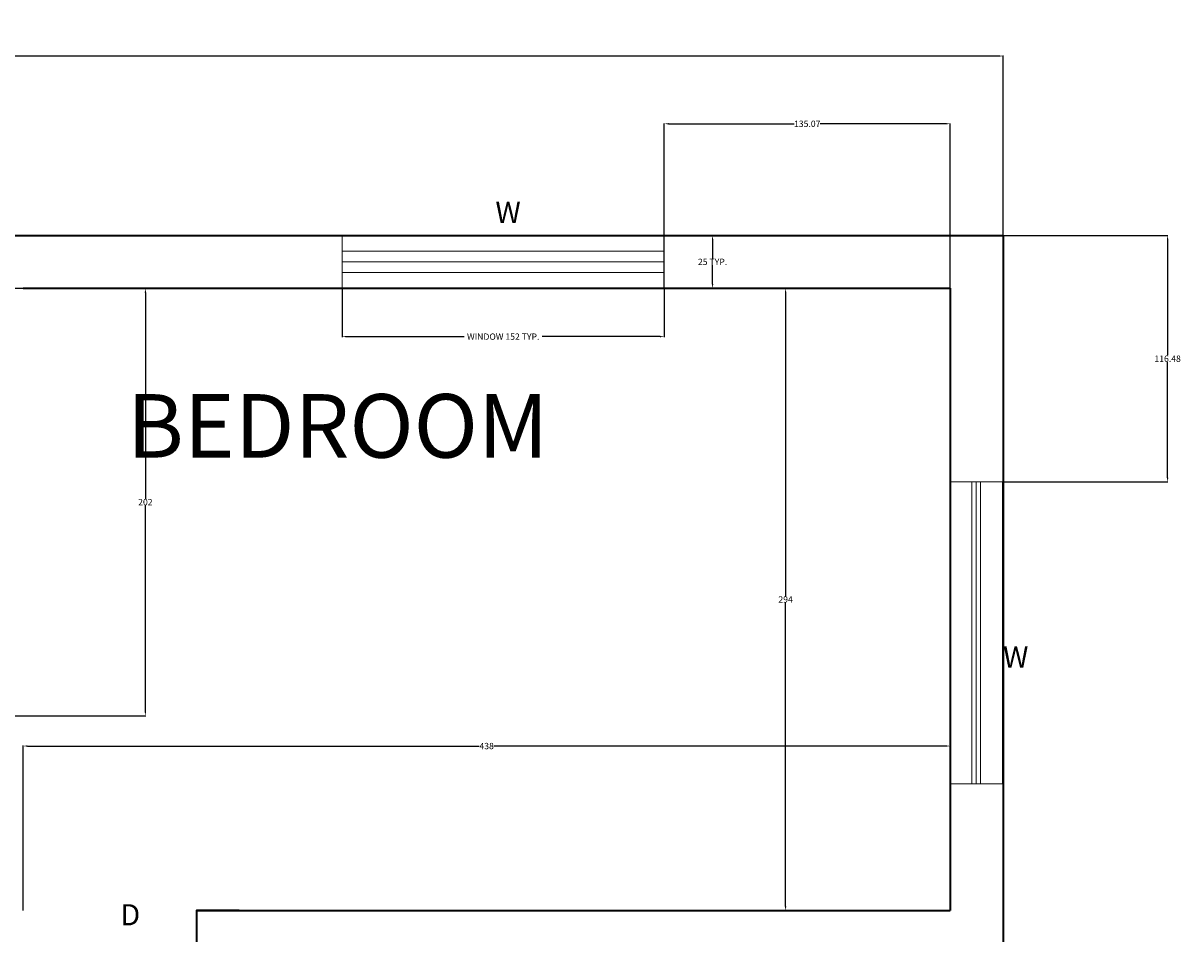
# Model space of a CAD drawing. Units: centimetres. Extents: x -121 to 3851, y -16 to 1180.
# Tile 16 of 16: x 3304 to 3851, y 582 to 1012. Entities that reach past the tile are written whole.
import ezdxf

# ---------------------------------------------------------------- set-up
doc = ezdxf.new("R2010")
doc.units = ezdxf.units.CM
doc.header["$MEASUREMENT"] = 0
for name, color, linetype, lineweight in [('A-ANNO-DIMS', 2, 'Continuous', 18), ('A-ANNO-IDEN', 3, 'Continuous', 13), ('A-AREA-IDEN', 3, 'Continuous', 18), ('A-GLAZ', 4, 'Continuous', 18), ('A-WALL', 7, 'Continuous', 35)]:
    doc.layers.add(name, color=color, linetype=linetype, lineweight=lineweight)
doc.styles.get("Standard").update_dxf_attribs({"font": 'arial.ttf'})
doc.dimstyles.get("Standard").update_dxf_attribs({"dimtxt": 3, "dimasz": 2, "dimexe": 0.18, "dimexo": 0.0625, "dimgap": 0.09, "dimtad": 0, "dimtih": 1, "dimtoh": 1, "dimdec": 0, "dimzin": 0, "dimdsep": 46, "dimtxsty": 'Standard', "dimcen": 0.09, "dimadec": 0, "dimazin": 0, "dimtfac": 1, "dimtdec": 0, "dimtofl": 0, "dimtmove": 0, "dimatfit": 3, "dimfxl": 1, "dimtolj": 1, "dimtzin": 0, "dimarcsym": 0})

# ---------------------------------------------------------------- blocks, each defined once
blk = doc.blocks.new('*D16')
at = {"layer": 'A-ANNO-DIMS', "color": 0, "lineweight": -2, "transparency": 16777216}
for p, q in [((2411.26, 911.79), (2411.26, 996.66)), ((2413.26, 996.48), (3045.8, 996.48)), ((3765.26, 996.48), (3132.73, 996.48)), ((3767.26, 911.79), (3767.26, 996.66))]:
    blk.add_line(p, q, dxfattribs=at)
at = {"layer": 'A-ANNO-DIMS', "color": 0, "transparency": 16777216}
for points in [[(2413.26, 996.81), (2413.26, 996.14), (2411.26, 996.48)], [(3765.26, 996.81), (3765.26, 996.14), (3767.26, 996.48)]]:
    blk.add_solid(points, dxfattribs=at)
at = {"layer": 'Defpoints', "color": 0, "transparency": 16777216}
for p in [(3767.26, 996.48), (2411.26, 911.72), (3767.26, 911.72)]:
    blk.add_point(p, dxfattribs=at)
at = {"layer": 'A-ANNO-DIMS', "color": 0, "transparency": 16777216, "insert": (3089.26, 996.48), "char_height": 3, "attachment_point": 5}
blk.add_mtext('\\A1;{\\H10x;1356}', dxfattribs=at)
blk = doc.blocks.new('WIN-152CM')
for p, q in [((0, 17.5), (152.19, 17.5)), ((0, 12.5), (152.19, 12.5)), ((0, 7.5), (152.19, 7.5))]:
    blk.add_line(p, q)
blk.add_lwpolyline([(0, 25), (152.19, 25), (152.19, 0), (0, 0)], close=True)
blk = doc.blocks.new('WIN-143CM')
for p, q in [((0, 14.5), (142.63, 14.5)), ((0, 12.5), (142.63, 12.5)), ((0, 10.5), (142.63, 10.5))]:
    blk.add_line(p, q)
blk.add_lwpolyline([(0, 25), (142.63, 25), (142.63, 0), (0, 0)], close=True)
blk = doc.blocks.new('*D27')
at = {"layer": 'A-ANNO-DIMS', "color": 0, "lineweight": -2, "transparency": 16777216}
for p, q in [((3455, 886.66), (3455, 863.71)), ((3607.19, 886.66), (3607.19, 863.71)), ((3457, 863.89), (3512.7, 863.89)), ((3605.19, 863.89), (3549.49, 863.89))]:
    blk.add_line(p, q, dxfattribs=at)
at = {"layer": 'A-ANNO-DIMS', "color": 0, "transparency": 16777216}
for points in [[(3457, 864.23), (3457, 863.56), (3455, 863.89)], [(3605.19, 864.23), (3605.19, 863.56), (3607.19, 863.89)]]:
    blk.add_solid(points, dxfattribs=at)
at = {"layer": 'Defpoints', "color": 0, "transparency": 16777216}
for p in [(3455, 886.72), (3607.19, 886.72), (3607.19, 863.89)]:
    blk.add_point(p, dxfattribs=at)
at = {"layer": 'A-ANNO-DIMS', "color": 0, "transparency": 16777216, "insert": (3531.09, 863.89), "char_height": 3, "attachment_point": 5}
blk.add_mtext('\\A1;WINDOW 152 TYP.', dxfattribs=at)
blk = doc.blocks.new('*D28')
at = {"layer": 'A-ANNO-DIMS', "color": 0, "lineweight": -2, "transparency": 16777216}
for p, q in [((3607.25, 911.72), (3630.2, 911.72)), ((3630.02, 909.72), (3630.02, 900.84)), ((3630.02, 888.72), (3630.02, 897.6)), ((3607.25, 886.72), (3630.2, 886.72))]:
    blk.add_line(p, q, dxfattribs=at)
at = {"layer": 'A-ANNO-DIMS', "color": 0, "transparency": 16777216}
for points in [[(3629.68, 909.72), (3630.35, 909.72), (3630.02, 911.72)], [(3629.68, 888.72), (3630.35, 888.72), (3630.02, 886.72)]]:
    blk.add_solid(points, dxfattribs=at)
at = {"layer": 'Defpoints', "color": 0, "transparency": 16777216}
for p in [(3607.19, 911.72), (3630.02, 911.72), (3607.19, 886.72)]:
    blk.add_point(p, dxfattribs=at)
at = {"layer": 'A-ANNO-DIMS', "color": 0, "transparency": 16777216, "insert": (3630.02, 899.22), "char_height": 3, "attachment_point": 5}
blk.add_mtext('\\A1;25 TYP.', dxfattribs=at)
blk = doc.blocks.new('*D69')
at = {"layer": 'A-ANNO-DIMS', "color": 0, "lineweight": -2, "transparency": 16777216}
for p, q in [((3284.33, 886.72), (3362.19, 886.72)), ((3362.01, 884.72), (3362.01, 787.34)), ((3362.01, 686.72), (3362.01, 784.1)), ((3284.33, 684.72), (3362.19, 684.72))]:
    blk.add_line(p, q, dxfattribs=at)
at = {"layer": 'A-ANNO-DIMS', "color": 0, "transparency": 16777216}
for points in [[(3361.68, 884.72), (3362.35, 884.72), (3362.01, 886.72)], [(3361.68, 686.72), (3362.35, 686.72), (3362.01, 684.72)]]:
    blk.add_solid(points, dxfattribs=at)
at = {"layer": 'Defpoints', "color": 0, "transparency": 16777216}
for p in [(3284.26, 886.72), (3284.26, 684.72), (3362.01, 684.72)]:
    blk.add_point(p, dxfattribs=at)
at = {"layer": 'A-ANNO-DIMS', "color": 0, "transparency": 16777216, "insert": (3362.01, 785.72), "char_height": 3, "attachment_point": 5}
blk.add_mtext('\\A1;202', dxfattribs=at)
blk = doc.blocks.new('*D70')
at = {"layer": 'A-ANNO-DIMS', "color": 0, "lineweight": -2, "transparency": 16777216}
for p, q in [((3767.33, 911.72), (3845.19, 911.72)), ((3845.01, 909.72), (3845.01, 855.11)), ((3845.01, 797.25), (3845.01, 851.86)), ((3767.14, 795.25), (3845.19, 795.25))]:
    blk.add_line(p, q, dxfattribs=at)
at = {"layer": 'A-ANNO-DIMS', "color": 0, "transparency": 16777216}
for points in [[(3844.68, 909.72), (3845.35, 909.72), (3845.01, 911.72)], [(3844.68, 797.25), (3845.35, 797.25), (3845.01, 795.25)]]:
    blk.add_solid(points, dxfattribs=at)
at = {"layer": 'Defpoints', "color": 0, "transparency": 16777216}
for p in [(3767.26, 911.72), (3767.07, 795.25), (3845.01, 795.25)]:
    blk.add_point(p, dxfattribs=at)
at = {"layer": 'A-ANNO-DIMS', "color": 0, "transparency": 16777216, "insert": (3845.01, 853.48), "char_height": 3, "attachment_point": 5}
blk.add_mtext('\\A1;116.48', dxfattribs=at)
blk = doc.blocks.new('*D71')
at = {"layer": 'A-ANNO-DIMS', "color": 0, "lineweight": -2, "transparency": 16777216}
for p, q in [((3607.19, 886.79), (3607.19, 964.65)), ((3609.19, 964.47), (3668.55, 964.47)), ((3740.26, 964.47), (3680.9, 964.47)), ((3742.26, 886.79), (3742.26, 964.65))]:
    blk.add_line(p, q, dxfattribs=at)
at = {"layer": 'A-ANNO-DIMS', "color": 0, "transparency": 16777216}
for points in [[(3609.19, 964.81), (3609.19, 964.14), (3607.19, 964.47)], [(3740.26, 964.81), (3740.26, 964.14), (3742.26, 964.47)]]:
    blk.add_solid(points, dxfattribs=at)
at = {"layer": 'Defpoints', "color": 0, "transparency": 16777216}
for p in [(3742.26, 964.47), (3607.19, 886.72), (3742.26, 886.72)]:
    blk.add_point(p, dxfattribs=at)
at = {"layer": 'A-ANNO-DIMS', "color": 0, "transparency": 16777216, "insert": (3674.73, 964.47), "char_height": 3, "attachment_point": 5}
blk.add_mtext('\\A1;135.07', dxfattribs=at)
blk = doc.blocks.new('*D81')
at = {"layer": 'A-ANNO-DIMS', "color": 0, "lineweight": -2, "transparency": 16777216}
for p, q in [((3304.26, 592.79), (3304.26, 670.65)), ((3306.26, 670.47), (3519.8, 670.47)), ((3740.26, 670.47), (3526.73, 670.47)), ((3742.26, 592.79), (3742.26, 670.65))]:
    blk.add_line(p, q, dxfattribs=at)
at = {"layer": 'A-ANNO-DIMS', "color": 0, "transparency": 16777216}
for points in [[(3306.26, 670.81), (3306.26, 670.14), (3304.26, 670.47)], [(3740.26, 670.81), (3740.26, 670.14), (3742.26, 670.47)]]:
    blk.add_solid(points, dxfattribs=at)
at = {"layer": 'Defpoints', "color": 0, "transparency": 16777216}
for p in [(3742.26, 670.47), (3304.26, 592.72), (3742.26, 592.72)]:
    blk.add_point(p, dxfattribs=at)
at = {"layer": 'A-ANNO-DIMS', "color": 0, "transparency": 16777216, "insert": (3523.26, 670.47), "char_height": 3, "attachment_point": 5}
blk.add_mtext('\\A1;438', dxfattribs=at)
blk = doc.blocks.new('*D82')
at = {"layer": 'A-ANNO-DIMS', "color": 0, "lineweight": -2, "transparency": 16777216}
for p, q in [((3742.2, 886.72), (3664.33, 886.72)), ((3664.51, 884.72), (3664.51, 741.34)), ((3664.51, 594.72), (3664.51, 738.1)), ((3742.2, 592.72), (3664.33, 592.72))]:
    blk.add_line(p, q, dxfattribs=at)
at = {"layer": 'A-ANNO-DIMS', "color": 0, "transparency": 16777216}
for points in [[(3664.18, 884.72), (3664.85, 884.72), (3664.51, 886.72)], [(3664.18, 594.72), (3664.85, 594.72), (3664.51, 592.72)]]:
    blk.add_solid(points, dxfattribs=at)
at = {"layer": 'Defpoints', "color": 0, "transparency": 16777216}
for p in [(3664.51, 886.72), (3742.26, 886.72), (3742.26, 592.72)]:
    blk.add_point(p, dxfattribs=at)
at = {"layer": 'A-ANNO-DIMS', "color": 0, "transparency": 16777216, "insert": (3664.51, 739.72), "char_height": 3, "attachment_point": 5}
blk.add_mtext('\\A1;294', dxfattribs=at)

msp = doc.modelspace()

# ---------------------------------------------------------------- linework, layer by layer
at = {"layer": 'A-WALL'}
for p, q in [((2736.2642, 911.7228), (3767.2642, 911.7228)), ((3767.2642, 911.7228), (3767.2642, 95.7228)), ((3304.2642, 886.7228), (3742.2642, 886.7228)), ((3742.2642, 886.7228), (3742.2642, 592.7228)), ((3386.2335, 592.7228), (3742.2642, 592.7228))]:
    msp.add_line(p, q, dxfattribs=at)
msp.add_lwpolyline([(3406.327, 592.7228), (3386.2335, 592.7228), (3386.2335, 415.7228)], dxfattribs=at)

# ---------------------------------------------------------------- block references
at = {"layer": 'A-GLAZ'}
msp.add_blockref('WIN-152CM', (3454.9993, 886.7227), dxfattribs=at)
at = {"layer": 'A-GLAZ', "rotation": 89.99999999999976}
msp.add_blockref('WIN-143CM', (3767.0732, 652.6168), dxfattribs=at)

# ---------------------------------------------------------------- texts
at = {"layer": 'A-ANNO-IDEN', "char_height": 10, "attachment_point": 1}
for s, insert in [('W', (3527.3985, 927.6121)), ('W', (3767.2642, 717.5214)), ('D', (3350.1824, 595.7422))]:
    msp.add_mtext_dynamic_manual_height_columns(s, width=55.718495, gutter_width=1, heights=[0], dxfattribs=dict(at, insert=insert))
at = {"layer": 'A-AREA-IDEN', "insert": (3353.2806, 836.7321), "char_height": 30, "attachment_point": 1}
msp.add_mtext_dynamic_manual_height_columns('BEDROOM', width=248.976965, gutter_width=1, heights=[0], dxfattribs=at)

# ---------------------------------------------------------------- dimensions: what is measured, and where the dimension line sits
at = {"layer": 'A-ANNO-DIMS'}
for base, p1, p2, text, override, picture, middle in [((3767.2642, 996.4769), (2411.2642, 911.7228), (3767.2642, 911.7228), '{\\H10x;<>}', {"dimclrd": 0, "dimclre": 0, "dimclrt": 0}, '*D16', (3089.2642, 996.4769)), ((3607.1897, 863.8943), (3454.9995, 886.7228), (3607.1897, 886.7228), 'WINDOW <> TYP.', {"dimdec": 0, "dimlfac": 1, "dimrnd": 0, "dimzin": 0, "dimdsep": 46, "dimlunit": 2}, '*D27', (3531.0946, 863.8943))]:
    dim = msp.add_linear_dim(base=base, p1=p1, p2=p2, text=text, dimstyle='Standard', override=override, dxfattribs=at)
    dim.commit()
    dim.dimension.update_dxf_attribs({"geometry": picture, "text_midpoint": middle})
for base, p1, p2, override, picture, middle in [((3742.2642, 964.4728), (3607.1897, 886.7228), (3742.2642, 886.7228), {"dimdec": 2, "dimlfac": 1, "dimrnd": 0, "dimzin": 0, "dimdsep": 46, "dimlunit": 2}, '*D71', (3674.727, 964.4728)), ((3742.2642, 670.4728), (3304.2642, 592.7228), (3742.2642, 592.7228), {"dimdec": 0, "dimlfac": 1, "dimrnd": 0, "dimzin": 0, "dimdsep": 46, "dimlunit": 2}, '*D81', (3523.2642, 670.4728))]:
    dim = msp.add_linear_dim(base=base, p1=p1, p2=p2, dimstyle='Standard', override=override, dxfattribs=at)
    dim.commit()
    dim.dimension.update_dxf_attribs({"geometry": picture, "text_midpoint": middle})
dim = msp.add_linear_dim(base=(3630.0183, 911.7228), p1=(3607.1897, 886.7228), p2=(3607.1897, 911.7228), angle=90, text='<> TYP.', dimstyle='Standard', override={"dimdec": 0, "dimlfac": 1, "dimrnd": 0, "dimzin": 0, "dimdsep": 46, "dimlunit": 2}, dxfattribs=at)
dim.commit()
dim.dimension.update_dxf_attribs({"geometry": '*D28', "text_midpoint": (3630.0183, 899.2228)})
for base, p1, p2, angle, override, picture, middle in [((3845.0142, 795.245), (3767.2642, 911.7228), (3767.0731, 795.245), 90, {"dimdec": 2, "dimlfac": 1, "dimrnd": 0, "dimzin": 0, "dimdsep": 46, "dimlunit": 2}, '*D70', (3845.0142, 853.4839)), ((3362.0142, 684.7228), (3284.2642, 886.7228), (3284.2642, 684.7228), 270, {"dimdec": 0, "dimlfac": 1, "dimrnd": 0, "dimzin": 0, "dimdsep": 46, "dimlunit": 2}, '*D69', (3362.0142, 785.7228)), ((3664.5142, 886.7228), (3742.2642, 592.7228), (3742.2642, 886.7228), 90, {"dimdec": 0, "dimlfac": 1, "dimrnd": 0, "dimzin": 0, "dimdsep": 46, "dimlunit": 2}, '*D82', (3664.5142, 739.7228))]:
    dim = msp.add_linear_dim(base=base, p1=p1, p2=p2, angle=angle, dimstyle='Standard', override=override, dxfattribs=at)
    dim.commit()
    dim.dimension.update_dxf_attribs({"geometry": picture, "text_midpoint": middle})

doc.saveas('drawing.dxf')
